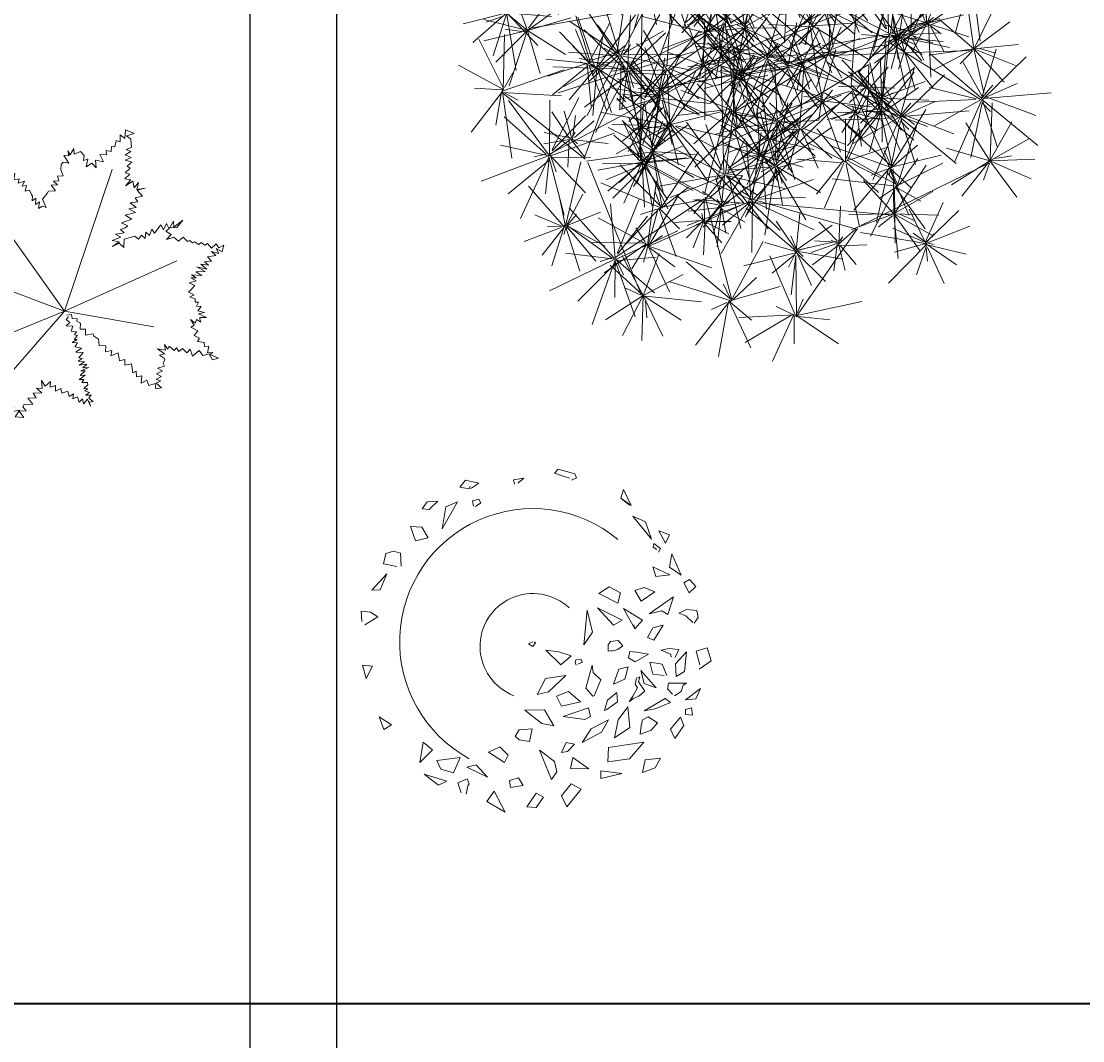
# Model space of a CAD drawing. Units: inches. Extents: x 8049 to 8459, y 820 to 1350.
# Tile 9 of 25: x 8132 to 8157, y 853 to 877. Entities that reach past the tile are written whole.
import ezdxf

# ---------------------------------------------------------------- set-up
doc = ezdxf.new("R2010")
doc.units = ezdxf.units.IN
doc.header["$MEASUREMENT"] = 0
for name, color, linetype, lineweight in [('A-ANNO-DIMS', 2, 'Continuous', 18), ('C-SITE-WALL', 7, 'Continuous', 35), ('zelen', 69, 'Continuous', 13)]:
    doc.layers.add(name, color=color, linetype=linetype, lineweight=lineweight)
doc.styles.get("Standard").update_dxf_attribs({"font": 'arial.ttf'})
doc.dimstyles.get("Standard").update_dxf_attribs({"dimtxt": 0.18, "dimasz": 0.18, "dimexe": 0.18, "dimexo": 0.0625, "dimgap": 0.09, "dimtad": 0, "dimtih": 1, "dimtoh": 1, "dimdec": 4, "dimzin": 0, "dimdsep": 46, "dimtxsty": 'Standard', "dimcen": 0.09, "dimadec": 0, "dimazin": 0, "dimtfac": 1, "dimtdec": 4, "dimtofl": 0, "dimtmove": 0, "dimatfit": 3, "dimfxl": 1, "dimtolj": 1, "dimtzin": 0, "dimarcsym": 0})

# ---------------------------------------------------------------- blocks, each defined once
blk = doc.blocks.new('z_96')
for p, q in [((-279.8, 149.9), (-254.2, 304.5)), ((-277.5, 143.8), (-209, 319.2)), ((0.6, 181.7), (29.5, 299.6)), ((-279.3, 139.9), (-326.8, 270.9)), ((-2.3, 183.5), (-55.4, 292.1)), ((5.7, 184.9), (91.8, 284.8)), ((-282.5, 143.4), (-440.4, 263.7)), ((1.7, 182.4), (-92.5, 262.1)), ((3.6, 188.7), (58.7, 265.3)), ((395.6, 94.6), (438.6, 246.5)), ((-276.5, 141.1), (-146.8, 221.3)), ((-9.6, 182.8), (-129.6, 222.9)), ((393.4, 89.6), (354, 209.2)), ((-292.1, 134.2), (-430.8, 180.4)), ((-5.7, 186.4), (-99.8, 114.3)), ((-4.6, 181.6), (-86.6, 72.3)), ((-0.6, 184.6), (125.7, 194.4)), ((1.5, 182.8), (69.9, 77.5)), ((9.8, 182.3), (88, 114.6)), ((393.4, 89.6), (479.1, 181.8)), ((-280.1, 150.3), (-304, 174)), ((-260.4, 142.3), (-97.9, 156.1)), ((-4.6, -3.2), (0.8, 176.4)), ((393.4, 89.6), (284.7, 153.1)), ((-283.2, 138.5), (-471.2, 114.9)), ((-279.1, 142.3), (-397.9, 16.9)), ((-285.6, 136.6), (-375, 92.2)), ((-277.6, 139.7), (-313.4, -1.1)), ((-279.1, 135.4), (-307.4, 99.5)), ((-278.4, 130.6), (-221.9, 40)), ((-277.5, 137.2), (-129.1, 19.3)), ((-17.8, -5.6), (-274.7, 141.8)), ((-263.2, 140.3), (-131, 113.5)), ((393.4, 89.6), (514.5, 123.6)), ((393.4, 89.6), (273.9, 50.1)), ((393.4, 89.6), (293.9, 12.5)), ((393.4, 89.6), (493.5, 13.4)), ((393.4, 89.6), (516.7, 64.5)), ((393.4, 89.6), (442.6, -26.2)), ((409.2, 93.4), (456.4, 89)), ((-71.7, -35.5), (-42.1, 65.4)), ((0, 0), (389.1, 84.4)), ((391.3, 83.5), (363.2, 41.9)), ((-74.7, -24.6), (-111.9, 37.5)), ((164.1, -89.9), (142.7, 11.7)), ((163.4, -89), (238.9, 7.6)), ((-237.5, -199.4), (-267, -22)), ((-10.4, -6), (-235.7, -205.3)), ((-65.2, -32.9), (-135.5, -11.4)), ((-80, -28.7), (-89.9, -20)), ((-16, -6.1), (-74.7, -37.4)), ((-68.1, -28.4), (-55.8, -19.3)), ((-5, -18.9), (163.8, -91.6)), ((159.3, -86.3), (85.5, -28.7)), ((167, -88.4), (276, -24.7)), ((-234, -202.3), (-196.3, -40.6)), ((-75, -39.2), (-157.1, -75.4)), ((-74, -33), (-152.4, -40.5)), ((-76.2, -35.8), (-103.5, -105.8)), ((-72.5, -35.1), (-71.9, -112)), ((-70.4, -41.1), (3.7, -57.1)), ((-69.9, -39.6), (-38.4, -102.6)), ((163.4, -86.5), (137.7, -55.7)), ((165.3, -92), (295.7, -74)), ((168.3, -88.4), (194, -71.5)), ((167.1, -94.6), (37.3, -175)), ((161.1, -92.4), (74, -95.2)), ((163.6, -101.8), (119, -170.9)), ((164.5, -93.4), (157.3, -141.4)), ((160.4, -93), (267.6, -148.2)), ((164.2, -92.2), (234.3, -170.2)), ((166.9, -90.5), (187.1, -100.1)), ((167, -104.1), (188, -212.9)), ((-237.4, -199.3), (-392.1, -169)), ((-246.4, -194), (-283.1, -163.8)), ((-231, -196), (-205.2, -161.9)), ((-242.3, -196.3), (-391.5, -241.3)), ((-242.2, -199.4), (-329.5, -310.3)), ((-241, -201.7), (-259.1, -277.3)), ((-242.2, -201.7), (-47.9, -207.3)), ((-236.2, -200.9), (-139.2, -306.8)), ((-230.8, -205.8), (-146.5, -236))]:
    blk.add_line(p, q)
blk = doc.blocks.new('сосна 1')
for p, rotation in [((317.7, 388.3), 121.1570021628385), ((-412.6, 386.5), 205.4822314301707), ((-117.1, 122.3), 55.05972244949475), ((-136.5, 361.1), 177.7388340989747), ((-351.5, 121.7), 257.3134436407499), ((-143.1, -5.5), 121.1570021628385), ((285.8, 9.1), 60.73020616460848), ((-343.1, -101.5), 57.88453704712605), ((234.4, -65.1), 73.8676290404427), ((-274, 161.3), 177.7388340989747), ((173.8, 17), 349.7944254651076), ((326.9, 45.9), 177.7388340989747), ((98.1, -4.6), 177.7388340989747), ((-175.3, -367), 63.19571700542104), ((-502.4, -282.3), 279.7984529833926), ((-48.9, -393.6), 342.5348703671633), ((260.9, -458.6), 13.72293452966709)]:
    blk.add_blockref('z_96', p, dxfattribs=dict(rotation=rotation))
blk = doc.blocks.new('z_85')
for p, q in [((168.5, 483.9), (169.7, 507.5)), ((169.7, 507.5), (194.7, 497.5)), ((140.4, 459.9), (144.1, 478.3)), ((144.1, 478.3), (154.8, 474.2)), ((154.8, 474.2), (155.6, 493.8)), ((155.6, 493.8), (168.5, 483.9)), ((194.7, 497.5), (173, 491.4)), ((173, 491.4), (185.2, 481.2)), ((185.2, 481.2), (186.9, 458.5)), ((8.4, 449), (15.4, 438)), ((11.7, 434.9), (8.4, 449)), ((15.4, 438), (25.6, 455.6)), ((25.6, 455.6), (26.4, 439.7)), ((26.4, 439.7), (44.1, 447.4)), ((44.1, 447.4), (54.4, 436.3)), ((116.1, 450.2), (130, 447.6)), ((116.6, 438), (116.1, 450.2)), ((130, 447.6), (130.9, 460.7)), ((130.9, 460.7), (140.4, 459.9)), ((185.1, 447.3), (169, 438)), ((186.9, 458.5), (172.1, 453.2)), ((172.1, 453.2), (185.1, 447.3)), ((-334.5, 433), (-320.5, 441.8)), ((-320.3, 426.3), (-334.5, 433)), ((-331, 417), (-320.3, 426.3)), ((-316.9, 407.2), (-331, 417)), ((-320.5, 441.8), (-312.2, 426.3)), ((-312.2, 426.3), (-302, 436.4)), ((-302, 436.4), (-292.5, 418.9)), ((-292.5, 418.9), (-282.7, 426.1)), ((-282.7, 426.1), (-277, 408.1)), ((-277, 408.1), (-266.3, 423.5)), ((-266.3, 423.5), (-258.7, 400.7)), ((-214.2, 421.3), (-198.5, 423)), ((-207.8, 406.4), (-214.2, 421.3)), ((-198.5, 423), (-198.2, 434.1)), ((-198.2, 434.1), (-192.6, 433.8)), ((-192.6, 433.8), (-192.5, 442.2)), ((-192.5, 442.2), (-183.3, 424.5)), ((-183.3, 424.5), (-173.3, 433.2)), ((-173.3, 433.2), (-176.4, 415.5)), ((-176.4, 415.5), (-165.1, 418.9)), ((-165.1, 418.9), (-166.4, 400.3)), ((-9.6, 410.9), (-3.8, 416.9)), ((-3.8, 416.9), (11.4, 414.5)), ((-2.1, 435.8), (11.7, 434.9)), ((11.4, 414.5), (-2.1, 435.8)), ((54.4, 436.3), (52.3, 421.7)), ((52.3, 421.7), (64.6, 426)), ((64.6, 426), (59.8, 403.9)), ((86.4, 422.5), (108.9, 418.4)), ((88.3, 401.4), (86.4, 422.5)), ((98.5, 438.8), (116.6, 438)), ((108.9, 418.4), (98.5, 438.8)), ((169, 438), (186.4, 430.3)), ((186.4, 430.3), (169.1, 422.7)), ((169.1, 422.7), (188.1, 417.5)), ((188.1, 417.5), (174.5, 406.5)), ((-325.3, 394.5), (-316.9, 407.2)), ((-309.5, 388.7), (-325.3, 394.5)), ((-317.2, 380.4), (-309.5, 388.7)), ((-258.7, 400.7), (-250.8, 414.2)), ((-250.8, 414.2), (-244.9, 399.8)), ((-244.9, 399.8), (-237.2, 410.8)), ((-237.2, 410.8), (-228.5, 393.9)), ((-228.5, 393.9), (-223.5, 408.6)), ((-223.5, 408.6), (-207.8, 406.4)), ((-166.4, 400.3), (-152.4, 402.8)), ((-152.4, 402.8), (-154.8, 385.2)), ((-10.8, 396), (-9.6, 410.9)), ((-4.1, 379.1), (-10.8, 396)), ((0, 0), (132.7, 397)), ((59.8, 403.9), (75.6, 414.2)), ((75.6, 414.2), (88.3, 401.4)), ((183.6, 400.7), (169.1, 387.1)), ((169.1, 387.1), (182.7, 383.5)), ((174.5, 406.5), (183.6, 400.7)), ((-305.1, 378.2), (-317.2, 380.4)), ((-309.5, 366.8), (-305.1, 378.2)), ((-299.2, 360.3), (-309.5, 366.8)), ((-305.9, 349.8), (-299.2, 360.3)), ((-154.8, 385.2), (-139.8, 385.6)), ((-139.8, 385.6), (-142, 367.5)), ((-142, 367.5), (-126.8, 370.7)), ((-126.8, 370.7), (-129.7, 358.9)), ((-129.7, 358.9), (-112.6, 364.1)), ((-112.6, 364.1), (-118.7, 349.7)), ((-31.2, 364.3), (-16.4, 364.7)), ((-19.6, 354.2), (-31.2, 364.3)), ((-19.9, 378.2), (-4.1, 379.1)), ((-16.4, 364.7), (-19.9, 378.2)), ((182.7, 383.5), (168.5, 371)), ((168.5, 371), (185.5, 367.5)), ((185.5, 367.5), (169.7, 351.3)), ((169.7, 351.3), (191.1, 364.1)), ((191.1, 364.1), (194, 345.3)), ((194, 345.3), (206.3, 360.8)), ((206.3, 360.8), (201.7, 341.2)), ((-292.6, 345.9), (-305.9, 349.8)), ((-305.3, 333.9), (-292.6, 345.9)), ((-288.9, 332.3), (-305.3, 333.9)), ((-296.8, 323.1), (-288.9, 332.3)), ((0, 0), (-245.8, 345.3)), ((-118.7, 349.7), (-106.5, 351.7)), ((-106.5, 351.7), (-110.4, 335.8)), ((-110.4, 335.8), (-98.6, 339.2)), ((-98.6, 339.2), (-92.9, 326.8)), ((-92.9, 326.8), (-89.6, 322.3)), ((-61.6, 314), (-48.8, 329.6)), ((-48.8, 329.6), (-45, 336.2)), ((-45, 336.2), (-26.1, 337)), ((-37.5, 352.7), (-19.6, 354.2)), ((-26.1, 337), (-37.5, 352.7)), ((201.7, 341.2), (224.8, 344.2)), ((224.8, 344.2), (203.2, 339.2)), ((203.2, 339.2), (217.5, 321.8)), ((-348.8, 287.5), (-334.3, 298.5)), ((-334.3, 298.5), (-333.4, 308.7)), ((-333.4, 308.7), (-315.2, 298.3)), ((-315.2, 298.3), (-314.9, 314.1)), ((-314.9, 314.1), (-305, 309.4)), ((-305, 309.4), (-300.9, 321)), ((-300.9, 321), (-284.3, 312.7)), ((-283.1, 324), (-296.8, 323.1)), ((-284.3, 312.7), (-283.1, 324)), ((-89.6, 322.3), (-91.1, 309)), ((-91.1, 309), (-80.4, 316.3)), ((-80.4, 316.3), (-81.2, 298.5)), ((-81.2, 298.5), (-70.2, 306.6)), ((-70.2, 306.6), (-73.6, 287.8)), ((-51.7, 290.2), (-61.6, 314)), ((204.7, 306.3), (183.1, 303.2)), ((183.1, 303.2), (199.8, 290.5)), ((217.5, 321.8), (196.8, 317.3)), ((196.8, 317.3), (204.7, 306.3)), ((-329.7, 291.9), (-348.8, 287.5)), ((-335.7, 285.2), (-329.7, 291.9)), ((-323.9, 282.5), (-335.7, 285.2)), ((-327.7, 273.4), (-323.9, 282.5)), ((-312.5, 269.8), (-327.7, 273.4)), ((-318.1, 260.9), (-312.5, 269.8)), ((-73.6, 287.8), (-62, 294.6)), ((-62, 294.6), (-51.7, 290.2)), ((198, 276.2), (169.3, 269.4)), ((169.3, 269.4), (187.9, 258.2)), ((199.8, 290.5), (179.5, 286.4)), ((179.5, 286.4), (198, 276.2)), ((-386.6, 246.8), (-370.9, 243.8)), ((-380.3, 234.1), (-386.6, 246.8)), ((-370.9, 243.8), (-362.5, 240.1)), ((-362.5, 240.1), (-355.4, 227.7)), ((-303.5, 257.1), (-318.1, 260.9)), ((-306.9, 250.2), (-303.5, 257.1)), ((-296.5, 245.4), (-306.9, 250.2)), ((-304.8, 236.9), (-296.5, 245.4)), ((187.9, 258.2), (158.6, 247.3)), ((158.6, 247.3), (176.5, 239.3)), ((176.5, 239.3), (169.1, 234)), ((251.2, 218.3), (269.1, 241.8)), ((269.1, 241.8), (276.1, 228.2)), ((276.1, 228.2), (284.6, 245.4)), ((284.6, 245.4), (292.5, 230.8)), ((292.5, 230.8), (304.2, 252.6)), ((304.2, 252.6), (305.4, 235.8)), ((305.4, 235.8), (330.6, 255.3)), ((330.6, 255.3), (314, 234.4)), ((-392, 203.9), (-391, 210.5)), ((-391, 210.5), (-375.1, 210.9)), ((-387.5, 216.4), (-377.3, 224.9)), ((-375.1, 210.9), (-387.5, 216.4)), ((-387.2, 228.2), (-380.3, 234.1)), ((-377.3, 224.9), (-387.2, 228.2)), ((-355.4, 227.7), (-347.7, 237.1)), ((-347.7, 237.1), (-340.1, 223.9)), ((-340.1, 223.9), (-331.2, 232.1)), ((-331.2, 232.1), (-323, 219.9)), ((-323, 219.9), (-314.9, 229.4)), ((-314.9, 229.4), (-308.7, 210.5)), ((-308.7, 210.5), (-301.4, 220.5)), ((-284, 230.8), (-304.8, 236.9)), ((-301.4, 220.5), (-296.2, 209.5)), ((-296.2, 209.5), (-288.7, 218.5)), ((-288.7, 218.5), (-282.8, 208)), ((-287.5, 222.7), (-284, 230.8)), ((-267.9, 221.3), (-287.5, 222.7)), ((-282.8, 208), (-278.3, 215.3)), ((-278.3, 215.3), (-269.6, 197)), ((-272.7, 208.1), (-267.9, 221.3)), ((-249.1, 208.6), (-272.7, 208.1)), ((-252.6, 191.1), (-249.1, 208.6)), ((166.6, 220), (142.5, 215.8)), ((142.5, 215.8), (157.5, 207.7)), ((169.1, 234), (156.5, 228.6)), ((156.5, 228.6), (166.6, 220)), ((166.1, 202.2), (195.8, 210)), ((195.8, 210), (206.3, 202.3)), ((206.3, 202.3), (214.9, 212.7)), ((214.9, 212.7), (225, 203.7)), ((225, 203.7), (227.4, 221.4)), ((227.4, 221.4), (237.6, 211.9)), ((237.6, 211.9), (244, 229.6)), ((244, 229.6), (251.2, 218.3)), ((291.9, 231.3), (282.8, 224.3)), ((282.8, 224.3), (297.7, 215.3)), ((297.7, 215.3), (285.2, 201.4)), ((294, 233.8), (291.9, 231.3)), ((314, 234.4), (294, 233.8)), ((-547.4, 195.4), (-527.9, 192.6)), ((-544.7, 179.5), (-547.4, 195.4)), ((-524.7, 189.5), (-544.7, 179.5)), ((-528.5, 176.6), (-524.7, 189.5)), ((-527.9, 192.6), (-523, 206.4)), ((-523, 206.4), (-504.7, 194.2)), ((-504.7, 194.2), (-496.5, 204.8)), ((-496.5, 204.8), (-486, 196.2)), ((-486, 196.2), (-473.8, 197.3)), ((-473.8, 197.3), (-470.6, 205)), ((-470.6, 205), (-459, 197.9)), ((-459, 197.9), (-453.2, 204.7)), ((-453.2, 204.7), (-441.7, 197.3)), ((-441.7, 197.3), (-436, 206.1)), ((-436, 206.1), (-423, 196.7)), ((-423, 196.7), (-417.9, 205.5)), ((-417.9, 205.5), (-411.3, 200.8)), ((-411.3, 200.8), (-403.9, 207.3)), ((-403.9, 207.3), (-392, 203.9)), ((-269.6, 197), (-261.6, 206.7)), ((-261.6, 206.7), (-252.6, 191.1)), ((157.5, 207.7), (133, 198.3)), ((133, 198.3), (152.7, 194.8)), ((152.7, 194.8), (134.2, 181.8)), ((134.2, 181.8), (152.3, 190.3)), ((152.3, 190.3), (165.5, 178.4)), ((165.5, 178.4), (166.1, 202.2)), ((285.2, 201.4), (305.7, 207.8)), ((305.7, 207.8), (318.4, 196.7)), ((318.4, 196.7), (331.5, 207.2)), ((331.5, 207.2), (343.4, 195.3)), ((343.4, 195.3), (349.2, 197.8)), ((349.2, 197.8), (357.1, 191.7)), ((357.1, 191.7), (363.4, 194)), ((363.4, 194), (375.4, 187.3)), ((375.4, 187.3), (381.6, 192.9)), ((381.6, 192.9), (391.6, 185.1)), ((391.6, 185.1), (399.5, 189.8)), ((399.5, 189.8), (410.7, 177.1)), ((410.7, 177.1), (423.8, 189)), ((423.8, 189), (430.9, 177.3)), ((430.9, 177.3), (445.2, 185.4)), ((445.2, 185.4), (440.2, 166.6)), ((-515.5, 177.6), (-528.5, 176.6)), ((-516.7, 167.9), (-515.5, 177.6)), ((-506.3, 173.2), (-516.7, 167.9)), ((-504.7, 162.4), (-506.3, 173.2)), ((-491.4, 165.7), (-504.7, 162.4)), ((-484.9, 140.6), (-491.4, 165.7)), ((0, 0), (-394.4, 149.4)), ((422.9, 156), (399.8, 152.7)), ((399.8, 152.7), (410.7, 140.5)), ((410.7, 167.7), (422.9, 156)), ((431.6, 161.5), (410.7, 167.7)), ((423.8, 175.6), (431.6, 161.5)), ((440.2, 166.6), (423.8, 175.6)), ((-472, 147), (-484.9, 140.6)), ((-466.4, 131.1), (-472, 147)), ((-447.4, 143.9), (-466.4, 131.1)), ((-446.4, 127.5), (-447.4, 143.9)), ((-431.2, 136.1), (-446.4, 127.5)), ((-433.6, 116.8), (-432.5, 124.7)), ((-432.5, 124.7), (-431.2, 136.1)), ((0, 0), (313.9, 140.8)), ((370, 124.5), (392.9, 111.3)), ((397.4, 117.9), (370, 124.5)), ((380.7, 131.9), (397.4, 117.9)), ((402.3, 129), (380.7, 131.9)), ((410.7, 140.5), (391.1, 138)), ((391.1, 138), (402.3, 129)), ((-456.8, 97.3), (-437.9, 103.7)), ((-452.6, 88.2), (-456.8, 97.3)), ((-447.3, 109), (-420.9, 115.7)), ((-437.9, 103.7), (-447.3, 109)), ((-420.9, 115.7), (-433.6, 116.8)), ((367.3, 93.6), (352.7, 93.5)), ((352.7, 93.5), (367.5, 85.5)), ((354.4, 102.3), (367.3, 93.6)), ((384, 100.5), (354.4, 102.3)), ((392.9, 111.3), (367, 110.4)), ((367, 110.4), (384, 100.5)), ((-490.1, 61.5), (-485.7, 76.6)), ((-472.7, 67.7), (-490.1, 61.5)), ((-485.7, 76.6), (-461.1, 77.2)), ((-477.3, 56.2), (-472.7, 67.7)), ((-464.1, 63.3), (-477.3, 56.2)), ((-468.4, 52.6), (-464.1, 63.3)), ((-452, 61.1), (-468.4, 52.6)), ((-466.3, 86.6), (-452.6, 88.2)), ((-461.1, 77.2), (-466.3, 86.6)), ((-455.1, 51.2), (-452, 61.1)), ((-439, 59.8), (-455.1, 51.2)), ((-439.5, 47.5), (-439, 59.8)), ((355.3, 62.8), (346.4, 53.6)), ((367.5, 85.5), (348.2, 79.7)), ((348.2, 79.7), (364, 72.5)), ((364, 72.5), (355.3, 62.8)), ((-428.5, 56.1), (-439.5, 47.5)), ((-421.5, 42.4), (-428.5, 56.1)), ((-408.4, 49.5), (-421.5, 42.4)), ((-406.6, 37.3), (-408.4, 49.5)), ((-393.5, 46.8), (-406.6, 37.3)), ((-392.2, 37), (-393.5, 46.8)), ((-375.3, 43.4), (-392.2, 37)), ((-368.7, 27.4), (-375.3, 43.4)), ((-356.3, 36.3), (-368.7, 27.4)), ((-348.5, 20.8), (-356.3, 36.3)), ((-333.9, 32.3), (-348.5, 20.8)), ((-335.5, 21.5), (-333.9, 32.3)), ((346.4, 53.6), (362.3, 46.4)), ((362.3, 46.4), (350.4, 40.1)), ((350.4, 40.1), (365.4, 35.2)), ((365.4, 35.2), (364.6, 26)), ((-322.4, 29.1), (-335.5, 21.5)), ((-319.9, 12.2), (-322.4, 29.1)), ((-303.8, 20), (-319.9, 12.2)), ((0, 0), (-312.2, -125)), ((-297.7, 5.3), (-303.8, 20)), ((-284.2, 12.8), (-297.7, 5.3)), ((-282.8, 2.5), (-284.2, 12.8)), ((-266.1, 11.6), (-282.8, 2.5)), ((-268.5, 0.9), (-266.1, 11.6)), ((-245.2, 1.9), (-268.5, 0.9)), ((-258.6, 1.3), (-245.2, 1.9)), ((-256.6, -5.5), (-258.6, 1.3)), ((0, 0), (-163.1, -186)), ((0, 0), (249.7, -43.2)), ((364.6, 26), (373.9, 25.2)), ((373.9, 25.2), (368.8, 14.6)), ((368.8, 14.6), (381.5, 13.5)), ((381.5, 13.5), (372.3, 1.1)), ((372.3, 1.1), (390.8, -3.1)), ((-337, -39.8), (-335.4, -26.5)), ((-335.4, -26.5), (-320, -32.7)), ((-320, -32.7), (-316.6, -19.6)), ((-316.6, -19.6), (-303.5, -24.4)), ((-303.5, -24.4), (-299.1, -12.1)), ((-299.1, -12.1), (-288.4, -18.9)), ((-288.4, -18.9), (-284.9, -7.8)), ((-284.9, -7.8), (-270.6, -10.5)), ((-272, -3.8), (-256.6, -5.5)), ((-270.6, -10.5), (-272, -3.8)), ((11, -15.5), (4.4, -23.3)), ((4.4, -23.3), (14.2, -31.5)), ((19.4, -9.1), (6, -11.1)), ((20.6, -19.7), (19.4, -9.1)), ((34.5, -21), (20.6, -19.7)), ((33.9, -27.7), (34.5, -21)), ((44.7, -33.5), (33.9, -27.7)), ((352.1, -22.6), (362.5, -39.2)), ((365.2, -32.7), (352.1, -22.6)), ((368.7, -23.2), (365.2, -32.7)), ((380.7, -30.1), (368.7, -23.2)), ((390.8, -3.1), (374.2, -7.2)), ((374.2, -7.2), (396.2, -16.9)), ((378.3, -17.7), (377.9, -21.9)), ((377.9, -21.9), (380.7, -30.1)), ((396.2, -16.9), (378.3, -17.7)), ((-423.6, -64.7), (-418.1, -55.3)), ((-418.1, -55.3), (-406.6, -63.9)), ((-406.6, -63.9), (-402.1, -52.8)), ((-402.1, -52.8), (-387.5, -58.3)), ((-387.5, -58.3), (-386, -47.3)), ((-386, -47.3), (-378.3, -50.6)), ((-378.3, -50.6), (-371.8, -40.4)), ((-371.8, -40.4), (-358.3, -47.6)), ((-358.6, -35.2), (-337, -39.8)), ((-358.3, -47.6), (-358.6, -35.2)), ((14.2, -31.5), (3.8, -40.4)), ((3.8, -40.4), (23.3, -42)), ((23.3, -42), (17.8, -55.3)), ((17.8, -55.3), (33.3, -57.2)), ((33.3, -57.2), (27.6, -66.1)), ((43.2, -50.4), (44.7, -33.5)), ((57.8, -49.8), (43.2, -50.4)), ((57.8, -66.7), (57.8, -49.8)), ((362.5, -39.2), (352.9, -44.5)), ((352.9, -44.5), (372.4, -54.8)), ((372.4, -54.8), (362.2, -67.3)), ((-445.6, -85.2), (-442.8, -66.9)), ((-431.8, -81.7), (-445.6, -85.2)), ((-442.8, -66.9), (-423.6, -64.7)), ((-433, -93.3), (-431.8, -81.7)), ((-421.5, -86.1), (-433, -93.3)), ((-420.3, -102.3), (-421.5, -86.1)), ((35.4, -79.2), (20.9, -86.9)), ((20.9, -86.9), (36.1, -88.5)), ((35.8, -67.3), (26.2, -78.5)), ((26.2, -78.5), (35.4, -79.2)), ((27.6, -66.1), (35.8, -67.3)), ((36.1, -88.5), (28.2, -99.3)), ((79.4, -63.3), (57.8, -66.7)), ((80.6, -68.6), (79.4, -63.3)), ((95, -77.7), (80.6, -68.6)), ((96.5, -95.7), (95, -77.7)), ((362.2, -67.3), (377.4, -74.9)), ((377.4, -74.9), (371.4, -84.3)), ((371.4, -84.3), (390.2, -87.1)), ((390.2, -87.1), (391, -98.7)), ((-408.9, -93.6), (-420.3, -102.3)), ((-406.5, -108.7), (-408.9, -93.6)), ((-396.2, -96.8), (-406.5, -108.7)), ((-391.4, -111), (-396.2, -96.8)), ((-377.3, -108.5), (-391.4, -111)), ((-387.6, -122.5), (-377.3, -108.5)), ((28.2, -99.3), (46.8, -102.9)), ((31.9, -112.9), (31.3, -114)), ((31.3, -114), (51.4, -114.8)), ((46.8, -102.9), (31.9, -112.9)), ((51.4, -114.8), (39.8, -130.3)), ((114.9, -96.9), (96.5, -95.7)), ((113.9, -113.2), (114.9, -96.9)), ((131.6, -109.3), (113.9, -113.2)), ((129.5, -124.2), (131.6, -109.3)), ((150, -116), (129.5, -124.2)), ((153.5, -138.6), (150, -116)), ((259.9, -104.5), (278.9, -118.5)), ((281.6, -108.4), (259.9, -104.5)), ((278.9, -118.5), (264.8, -122.8)), ((279.1, -92.7), (281.6, -108.4)), ((288.4, -105.6), (279.1, -92.7)), ((292.3, -97.7), (288.4, -105.6)), ((306.3, -109.8), (292.3, -97.7)), ((312.3, -101.9), (306.3, -109.8)), ((319.1, -112.6), (312.3, -101.9)), ((329.4, -104.1), (319.1, -112.6)), ((341.7, -115.9), (329.4, -104.1)), ((350.6, -106.3), (341.7, -115.9)), ((357.5, -125.6), (350.6, -106.3)), ((375.9, -109.5), (357.5, -125.6)), ((386.6, -123.9), (375.9, -109.5)), ((403.8, -118.5), (386.6, -123.9)), ((391, -98.7), (403.6, -97.7)), ((403.6, -97.7), (399.4, -115.7)), ((399.4, -115.7), (414.2, -115.6)), ((413.1, -135.8), (403.8, -118.5)), ((414.2, -115.6), (406.2, -120.7)), ((-399.4, -144.9), (-386, -138.6)), ((-391.7, -153.5), (-399.4, -144.9)), ((-396.7, -133.3), (-378.8, -121.8)), ((-386, -138.6), (-396.7, -133.3)), ((-378.8, -121.8), (-387.6, -122.5)), ((49.4, -132), (38, -139.7)), ((38, -139.7), (55.7, -140.9)), ((39.8, -130.3), (49.4, -132)), ((55.7, -140.9), (40.8, -150.5)), ((40.8, -150.5), (61.7, -147.7)), ((61.7, -147.7), (51.2, -158.2)), ((168.2, -134.7), (153.5, -138.6)), ((168.7, -151.1), (168.2, -134.7)), ((187.2, -147), (168.7, -151.1)), ((190.4, -171.9), (187.2, -147)), ((264.8, -122.8), (279.4, -131.9)), ((280.4, -134.4), (275.3, -145.6)), ((275.3, -145.6), (279.5, -153.9)), ((279.4, -131.9), (280.4, -134.4)), ((406.2, -120.7), (430, -130.9)), ((430, -130.9), (413.1, -135.8)), ((-407.1, -178.7), (-394, -170.7)), ((-405.7, -161.9), (-391.7, -153.5)), ((-394, -170.7), (-405.7, -161.9)), ((57.7, -166.9), (43.5, -179.6)), ((67.9, -157.4), (45.5, -166.6)), ((45.5, -166.6), (57.7, -166.9)), ((51.2, -158.2), (67.9, -157.4)), ((199.5, -167.6), (190.4, -171.9)), ((201.2, -183.5), (199.5, -167.6)), ((273.9, -166.2), (257.2, -175.1)), ((257.2, -175.1), (270.6, -182.1)), ((279.5, -153.9), (259.5, -159.1)), ((259.5, -159.1), (273.9, -166.2)), ((-408.7, -191.2), (-407.1, -178.7)), ((-386.3, -183.7), (-408.7, -191.2)), ((-386.9, -194.2), (-386.3, -183.7)), ((-375, -185.4), (-386.9, -194.2)), ((-374.4, -200.4), (-375, -185.4)), ((-361, -190), (-374.4, -200.4)), ((-355.6, -205.5), (-361, -190)), ((-340.1, -188.9), (-355.6, -205.5)), ((-331, -204.2), (-340.1, -188.9)), ((-320.5, -190.1), (-331, -204.2)), ((-315.8, -206.4), (-320.5, -190.1)), ((-300.9, -199.4), (-315.8, -206.4)), ((-311, -217.5), (-300.9, -199.4)), ((-64.5, -193.4), (-63.1, -216.4)), ((-54.1, -209.7), (-64.5, -193.4)), ((-39.9, -196.5), (-54.1, -209.7)), ((-40.4, -212.5), (-39.9, -196.5)), ((-25.3, -207.7), (-40.4, -212.5)), ((-25.3, -223.8), (-25.3, -207.7)), ((57.1, -178.7), (40.5, -191.1)), ((40.5, -191.1), (53.9, -190.4)), ((43.5, -179.6), (57.1, -178.7)), ((53.9, -190.4), (47.9, -199)), ((47.9, -199), (63.4, -198.7)), ((65.1, -205.6), (53.6, -216.1)), ((63.4, -198.7), (65.1, -205.6)), ((215.4, -180.2), (201.2, -183.5)), ((214.3, -200.6), (215.4, -180.2)), ((229.7, -192.5), (214.3, -200.6)), ((235.5, -207.5), (229.7, -192.5)), ((253.5, -202), (235.5, -207.5)), ((255.4, -217.1), (253.5, -202)), ((270.6, -182.1), (255.6, -190.7)), ((255.6, -190.7), (268.7, -194.5)), ((268.7, -194.5), (256, -201.4)), ((256, -201.4), (270.6, -214.1)), ((-316.4, -230.7), (-301.2, -212.5)), ((-303, -227.7), (-316.4, -230.7)), ((-301.2, -212.5), (-311, -217.5)), ((-309.9, -238.3), (-303, -227.7)), ((-63.4, -228.2), (-87.9, -229.1)), ((-87.9, -229.1), (-79.8, -242)), ((-78.5, -215.2), (-63.4, -228.2)), ((-63.1, -216.4), (-78.5, -215.2)), ((-10.7, -215.8), (-25.3, -223.8)), ((-8.3, -228.6), (-10.7, -215.8)), ((8.9, -223.5), (-8.3, -228.6)), ((12.7, -238.7), (8.9, -223.5)), ((24.7, -230.5), (12.7, -238.7)), ((23, -244.8), (24.7, -230.5)), ((53.6, -216.1), (64.9, -216.9)), ((64.9, -216.9), (56, -222.4)), ((56, -222.4), (69.4, -226.9)), ((69.4, -226.9), (58.1, -234.3)), ((58.1, -234.3), (70.9, -234.4)), ((73.9, -233.5), (67.9, -243.4)), ((70.9, -234.4), (73.9, -233.5)), ((270.6, -214.1), (255.4, -217.1)), ((-298.3, -242.6), (-309.9, -238.3)), ((-305.3, -270.9), (-295, -254.3)), ((-304.7, -251.3), (-298.3, -242.6)), ((-295, -254.3), (-304.7, -251.3)), ((-166.3, -266.5), (-182.4, -271.4)), ((-151.2, -278.6), (-166.3, -266.5)), ((-113.1, -261.1), (-117.3, -267.5)), ((-88.9, -260), (-113.1, -261.1)), ((-79.8, -242), (-103.3, -242.6)), ((-103.3, -242.6), (-88.9, -260)), ((35.5, -238.8), (23, -244.8)), ((40.7, -254.5), (35.5, -238.8)), ((49.8, -244.9), (40.7, -254.5)), ((52.7, -259.2), (49.8, -244.9)), ((63.6, -245.9), (52.7, -259.2)), ((72.4, -265), (63.6, -245.9)), ((67.9, -243.4), (79.4, -252.4)), ((79.4, -252.4), (68.2, -253.9)), ((68.2, -253.9), (72.4, -265)), ((-290.1, -273.1), (-305.3, -270.9)), ((-294.6, -284.2), (-290.1, -273.1)), ((-277.1, -277.7), (-294.6, -284.2)), ((-264.9, -273), (-283.1, -288.1)), ((-283.1, -288.1), (-277.1, -277.7)), ((-264.3, -294.3), (-264.9, -273)), ((-256.6, -277.5), (-264.3, -294.3)), ((-254.5, -286.6), (-256.6, -277.5)), ((-239.6, -270.1), (-254.5, -286.6)), ((-228.6, -289.1), (-239.6, -270.1)), ((-220, -272), (-228.6, -289.1)), ((-197.9, -289.9), (-220, -272)), ((-199.2, -272), (-197.9, -289.9)), ((-184.2, -282), (-199.2, -272)), ((-182.4, -271.4), (-184.2, -282)), ((-142.3, -267.5), (-151.2, -278.6)), ((-144.6, -280.3), (-142.3, -267.5)), ((-126.2, -276.2), (-144.6, -280.3)), ((-138.9, -294.9), (-126.2, -276.2)), ((-114.3, -296.8), (-138.9, -294.9)), ((-107.8, -278), (-127.3, -279.2)), ((-127.3, -279.2), (-114.3, -296.8)), ((-117.3, -267.5), (-107.8, -278))]:
    blk.add_line(p, q)
blk = doc.blocks.new('z_66')
for p, q in [((83.2, 488.9), (72.7, 477.7)), ((72.7, 477.7), (96.4, 469.7)), ((129.8, 476.2), (83.2, 488.9)), ((134, 464.6), (129.8, 476.2)), ((-176.4, 458.5), (-191.7, 438.6)), ((-139.2, 449.4), (-176.4, 458.5)), ((-161.1, 434.6), (-139.2, 449.4)), ((-13.6, 463.6), (-42.5, 459.2)), ((-42.5, 459.2), (-39.3, 446.9)), ((-30.3, 449.4), (-13.6, 463.6)), ((96.4, 469.7), (114.5, 463.9)), ((114.5, 463.9), (114.5, 463.9)), ((120.4, 457.8), (134, 464.6)), ((-191.7, 438.6), (-165.6, 433.5)), ((-165.6, 433.5), (-163.6, 441.1)), ((-165.6, 433.5), (-165.6, 433.5)), ((265.2, 432.1), (258.2, 407.5)), ((287.4, 387.2), (265.2, 432.1)), ((-283.6, 397.7), (-297.2, 378.2)), ((-254, 399.9), (-283.6, 397.7)), ((-272.8, 380.7), (-254, 399.9)), ((-241.9, 321.7), (-199.1, 397.3)), ((-199.1, 397.3), (-231.4, 383.6)), ((-138.9, 404.9), (-156.9, 400.2)), ((-156.9, 400.2), (-153.8, 385.4)), ((-148.6, 384.7), (-133.3, 394.8)), ((-133.3, 394.8), (-138.9, 404.9)), ((258.2, 407.5), (287.4, 387.2)), ((258.2, 407.5), (281.9, 388.6)), ((281.9, 388.6), (281.9, 388.6)), ((-297.2, 378.2), (-277.7, 376)), ((-277.7, 376), (-272.8, 380.7)), ((-231.4, 383.6), (-241.9, 321.7)), ((344.2, 293.1), (292, 357.2)), ((292, 357.2), (326.8, 341.2)), ((-330.3, 328.9), (-298.6, 327.1)), ((-316, 288.8), (-330.3, 328.9)), ((-298.6, 327.1), (-280.8, 297.1)), ((326.8, 341.2), (344.2, 293.1)), ((-280.8, 297.1), (-316, 288.8)), ((383.1, 281.9), (364.4, 316.3)), ((364.4, 316.3), (394.6, 305.1)), ((394.6, 305.1), (383.1, 281.9)), ((350.8, 280.8), (348.7, 270.3)), ((348.7, 270.3), (358.8, 264.5)), ((369.2, 266.7), (350.8, 280.8)), ((-399.2, 252.6), (-405.8, 224)), ((-377.9, 259.1), (-399.2, 252.6)), ((-358.4, 254), (-377.9, 259.1)), ((-356, 217.5), (-358.4, 254)), ((358.8, 264.5), (358.8, 264.5)), ((363.3, 256.6), (369.2, 266.7)), ((400.9, 251.9), (393.9, 214.6)), ((426.6, 192.2), (400.9, 251.9)), ((-405.8, 224), (-368.2, 216.4)), ((-368.2, 216.4), (-368.2, 216.4)), ((348, 215.7), (356, 188.9)), ((395.3, 193.2), (348, 215.7)), ((393.9, 214.6), (426.6, 192.2)), ((-396.4, 196.1), (-438.1, 150.2)), ((-414.8, 150.9), (-396.4, 196.1)), ((356, 188.9), (395.3, 193.2)), ((450, 180.6), (434.3, 171.2)), ((467.7, 160.3), (450, 180.6)), ((-438.1, 150.2), (-414.8, 150.9)), ((225.2, 159.9), (197, 140.8)), ((256.8, 142.6), (225.2, 159.9)), ((323.6, 157.8), (297.5, 149.8)), ((297.5, 149.8), (314.6, 119.4)), ((352.9, 145.5), (323.6, 157.8)), ((434.3, 171.2), (449.6, 142.6)), ((449.6, 142.6), (467.7, 160.3)), ((197, 140.8), (249.5, 113.6)), ((249.5, 113.6), (256.8, 142.6)), ((314.6, 119.4), (352.9, 145.5)), ((336.9, 84.3), (405.8, 131.7)), ((405.8, 131.7), (389.8, 82.1)), ((-468.4, 91.6), (-466.3, 62.6)), ((-441.6, 89), (-468.4, 91.6)), ((164.3, 94.8), (154.2, -2.2)), ((178.9, 33.3), (164.3, 94.8)), ((193.1, 101.3), (238, 52.1)), ((261.7, 66.6), (193.1, 101.3)), ((265.2, 98.8), (297.2, 42.7)), ((318.8, 66.2), (265.2, 98.8)), ((372.7, 93), (336.9, 84.3)), ((389.8, 82.1), (372.7, 93)), ((441.6, 95.9), (420.7, 86.5)), ((470.5, 93.7), (441.6, 95.9)), ((474, 73.5), (470.5, 93.7)), ((-466.3, 62.6), (-466.3, 62.6)), ((-458.3, 53.9), (-421.1, 76)), ((-421.1, 76), (-441.6, 89)), ((238, 52.1), (261.7, 66.6)), ((297.2, 42.7), (318.8, 66.2)), ((420.7, 86.5), (440.2, 78.5)), ((440.2, 78.5), (459.7, 59.7)), ((459.7, 59.7), (459.7, 59.7)), ((463.2, 57.9), (474, 73.5)), ((154.2, -2.2), (178.9, 33.3)), ((297.2, 42.7), (294.1, 53.6)), ((347.3, 45.2), (332.7, 18.1)), ((376.9, 52.5), (347.3, 45.2)), ((350.8, 10.9), (376.9, 52.5)), ((11.8, 6.2), (0, 0)), ((0, 0), (12.2, -6.9)), ((12.2, -6.9), (19.1, 2.9)), ((19.1, 2.9), (15.7, 5.8)), ((229, 7.2), (223.1, -2.5)), ((250.6, 9.8), (229, 7.2)), ((263.4, -5.4), (250.6, 9.8)), ((332.7, 18.1), (350.8, 10.9)), ((84.6, -21.7), (48, -17)), ((48, -17), (90.1, -58.3)), ((119.4, -32.9), (84.6, -21.7)), ((223.1, -2.5), (222.7, -20.6)), ((222.7, -20.6), (234.2, -18.1)), ((233.2, -19.9), (249.9, -15.9)), ((234.2, -18.1), (234.2, -18.1)), ((249.9, -15.9), (263.4, -5.4)), ((282.9, -21.3), (279.1, -39.1)), ((302.1, -22.8), (282.9, -21.3)), ((298.6, -50.3), (335.8, -28.6)), ((335.8, -28.6), (302.1, -22.8)), ((393.6, -13), (371, -17)), ((371, -17), (383.5, -23.5)), ((383.5, -23.5), (396.7, -28.9)), ((420, -15.9), (393.6, -13)), ((396.7, -28.9), (398.5, -35.5)), ((410.3, -38), (420, -15.9)), ((442, -22.4), (411.3, -55.4)), ((436, -77.1), (442, -22.4)), ((499.7, -10.9), (468.8, -19.9)), ((468.8, -19.9), (478.8, -58.6)), ((510.9, -47), (499.7, -10.9)), ((-464.2, -59.3), (-436.4, -62.6)), ((-454.5, -96.3), (-464.2, -59.3)), ((90.1, -58.3), (119.4, -32.9)), ((131.9, -44.9), (130.2, -52.5)), ((130.2, -52.5), (132.9, -59.3)), ((146.5, -42.3), (131.9, -44.9)), ((138.2, -56.8), (151, -51)), ((151, -51), (146.5, -42.3)), ((177.8, -59), (160.1, -123.8)), ((181, -80.3), (177.8, -59)), ((279.1, -39.1), (298.6, -50.3)), ((339, -51), (347.7, -84.3)), ((374.1, -56.8), (339, -51)), ((386.3, -87.9), (374.1, -56.8)), ((398.5, -35.5), (399.5, -35.8)), ((411.3, -55.4), (412.7, -90.8)), ((477.5, -70.2), (510.9, -47)), ((478.8, -58.6), (478.8, -58.6)), ((-436.4, -62.6), (-454.5, -96.3)), ((104.1, -87.9), (47.7, -96.6)), ((56, -133.9), (104.1, -87.9)), ((202.2, -100.6), (181, -80.3)), ((252.6, -70.9), (237.7, -112.9)), ((278.4, -64), (252.6, -70.9)), ((269.7, -98.4), (278.4, -64)), ((314.2, -74.2), (356.7, -123)), ((323.3, -111.1), (314.2, -74.2)), ((347.7, -84.3), (379.7, -88.3)), ((379.7, -88.3), (379.7, -88.3)), ((412.7, -90.8), (436, -77.1)), ((47.7, -96.6), (24, -141.9)), ((183.7, -145.5), (202.2, -100.6)), ((237.7, -112.9), (269.7, -98.4)), ((301.7, -95.5), (297.9, -112.2)), ((297.9, -112.2), (304.5, -123)), ((310.8, -91.9), (301.7, -95.5)), ((307.6, -106), (310.8, -91.9)), ((325.4, -132.4), (307.6, -106)), ((356.7, -123), (323.3, -111.1)), ((391.2, -110), (388.4, -125.6)), ((391.2, -110), (393.2, -108.6)), ((441.3, -110), (391.2, -110)), ((427, -133.5), (432.9, -115.8)), ((432.9, -115.8), (441.3, -110)), ((24, -141.9), (56, -133.9)), ((111.4, -132.8), (78.3, -146.2)), ((78.3, -146.2), (92.2, -174.1)), ((145.1, -162.1), (111.4, -132.8)), ((160.1, -123.8), (179.6, -146.6)), ((179.6, -146.6), (183.7, -145.5)), ((247.1, -135.7), (220.6, -157)), ((249.2, -162.1), (247.1, -135.7)), ((291.6, -145.8), (281.2, -161.8)), ((304.5, -123), (291.6, -145.8)), ((293, -152.7), (308.3, -145.8)), ((308.3, -145.8), (325.4, -132.4)), ((356.7, -123), (356.7, -123)), ((356.7, -123), (356.7, -123)), ((388.4, -125.6), (402.3, -140.8)), ((402.3, -140.8), (402.3, -140.8)), ((407.9, -145.5), (427, -133.5)), ((480.9, -124.5), (439.2, -156)), ((467.7, -153.4), (480.9, -124.5)), ((92.2, -174.1), (145.1, -162.1)), ((220.6, -157), (212.6, -186)), ((219.2, -183.5), (249.2, -162.1)), ((277.4, -176.2), (250.2, -212.4)), ((283.3, -233.8), (277.4, -176.2)), ((281.2, -161.8), (293, -152.7)), ((382.5, -152.7), (323.3, -187.4)), ((353.9, -182), (396.7, -164.3)), ((396.7, -164.3), (382.5, -152.7)), ((439.2, -156), (467.7, -153.4)), ((-417.9, -204.1), (-405.1, -239.6)), ((-382.8, -226.5), (-417.9, -204.1)), ((44.5, -184.2), (-10.8, -184.9)), ((-10.8, -184.9), (36.9, -222.2)), ((71, -229.1), (44.5, -184.2)), ((168.1, -178.4), (96.7, -202.6)), ((96.7, -202.6), (157.6, -211.3)), ((157.6, -211.3), (173, -203.4)), ((173, -203.4), (168.1, -178.4)), ((212.6, -186), (219.2, -183.5)), ((334.1, -203.7), (318.4, -212.1)), ((323.3, -187.4), (353.9, -182)), ((360.2, -221.1), (334.1, -203.7)), ((425.3, -204.5), (396.7, -238.5)), ((434.3, -228), (425.3, -204.5)), ((438.5, -183.8), (456.2, -179.1)), ((438.5, -197.6), (438.5, -183.8)), ((458.7, -199), (438.5, -197.6)), ((456.2, -179.1), (458.7, -199)), ((-405.1, -239.6), (-382.8, -226.5)), ((36.9, -222.2), (71, -229.1)), ((223.8, -212.4), (175.4, -237.7)), ((204.3, -246.8), (223.8, -212.4)), ((250.2, -212.4), (240.1, -262.4)), ((240.1, -262.4), (283.3, -233.8)), ((314.6, -228.7), (311.8, -252.6)), ((318.4, -212.1), (314.6, -228.7)), ((342.8, -241.4), (360.2, -221.1)), ((409.2, -264.2), (434.3, -228)), ((-26.4, -240.3), (-37.6, -258.4)), ((-37.6, -258.4), (-25.8, -268.5)), ((10.1, -237.7), (-26.4, -240.3)), ((2.4, -273.2), (10.1, -237.7)), ((175.4, -237.7), (149.6, -276.1)), ((149.6, -276.1), (204.3, -246.8)), ((311.8, -252.6), (320.5, -249.3)), ((320.5, -249.3), (342.8, -241.4)), ((396.7, -238.5), (409.2, -264.2)), ((-295.1, -275), (-304.2, -331.5)), ((-304.2, -331.5), (-269, -296)), ((-269, -296), (-295.1, -275)), ((-80, -288), (-112.4, -302.5)), ((-56.7, -311.6), (-80, -288)), ((-25.8, -268.5), (2.4, -273.2)), ((-25.8, -268.5), (-25.8, -268.5)), ((-25.8, -268.5), (-25.8, -268.5)), ((105.1, -276.1), (91.9, -303.6)), ((128.8, -280.4), (105.1, -276.1)), ((108.6, -301.4), (128.8, -280.4)), ((223.8, -290.2), (221.3, -330)), ((322.2, -275), (223.8, -290.2)), ((282.2, -321.7), (322.2, -275)), ((-191.1, -317.4), (-256.8, -326.4)), ((-256.8, -326.4), (-245.7, -350.3)), ((-209.8, -360.4), (-191.1, -317.4)), ((-112.4, -302.5), (-67.5, -331.8)), ((-67.5, -331.8), (-56.7, -311.6)), ((30.6, -297.1), (72.7, -329.3)), ((64, -379.6), (30.6, -297.1)), ((91.9, -303.6), (108.6, -301.4)), ((117.3, -348.8), (124.2, -317.7)), ((124.2, -317.7), (168.8, -349.9)), ((221.3, -330), (282.2, -321.7)), ((325.7, -323.9), (318.4, -360.1)), ((368.9, -319.2), (325.7, -323.9)), ((354.3, -346.3), (368.9, -319.2)), ((-245.7, -350.3), (-209.8, -360.4)), ((-172.6, -344.9), (-146.9, -338.7)), ((-114.8, -372.7), (-172.6, -344.9)), ((-146.9, -338.7), (-114.8, -372.7)), ((72.7, -329.3), (79.3, -357.9)), ((168.8, -349.9), (117.3, -348.8)), ((201.8, -355), (202.2, -376.3)), ((261, -362.2), (201.8, -355)), ((318.4, -360.1), (354.3, -346.3)), ((-292, -364.4), (-252, -395.5)), ((-228.3, -383.9), (-292, -364.4)), ((-252, -395.5), (-228.3, -383.9)), ((-197.3, -388.3), (-171.2, -377.8)), ((-171.2, -377.8), (-166, -391.5)), ((-27.8, -374.5), (-52.9, -381.8)), ((-52.9, -381.8), (-50.8, -402)), ((-15.3, -396.2), (-27.8, -374.5)), ((79.3, -357.9), (64, -379.6)), ((202.2, -376.3), (261, -362.2)), ((-188.3, -416.9), (-197.3, -388.3)), ((-169.5, -396.6), (-174.7, -420.5)), ((-166, -391.5), (-169.5, -396.6)), ((-116.2, -441.1), (-96.4, -411.8)), ((-96.4, -411.8), (-65.8, -470.8)), ((-50.8, -402), (-15.3, -396.2)), ((91.9, -424.8), (119, -391.5)), ((146.9, -406.4), (106.8, -455.6)), ((119, -391.5), (146.9, -406.4)), ((-174.7, -420.5), (-174.7, -420.5)), ((-65.8, -470.8), (-116.2, -441.1)), ((21.6, -417.2), (-4.5, -455.6)), ((42.1, -428.8), (21.6, -417.2)), ((21.6, -458.1), (42.1, -428.8)), ((106.8, -455.6), (91.9, -424.8)), ((-4.5, -455.6), (21.6, -458.1))]:
    blk.add_line(p, q)
for centre, radius, start, end in [((11.8, 6.2), 372.3, 50.2118, 241.5185), ((12.2, -6.9), 147.8, 46.7611, 248.9067)]:
    blk.add_arc(centre, radius, start, end)
blk = doc.blocks.new('*D58')
at = {"layer": 'A-ANNO-DIMS', "color": 0, "lineweight": -2, "transparency": 16777216}
for p, q in [((8139.397, 1162.808), (8139.397, 820.091)), ((8175.397, 1162.808), (8175.397, 820.091)), ((8139.577, 820.271), (8157.179, 820.271)), ((8175.217, 820.271), (8157.616, 820.271))]:
    blk.add_line(p, q, dxfattribs=at)
at = {"layer": 'A-ANNO-DIMS', "color": 0, "transparency": 16777216}
for points in [[(8139.577, 820.301), (8139.577, 820.241), (8139.397, 820.271)], [(8175.217, 820.301), (8175.217, 820.241), (8175.397, 820.271)]]:
    blk.add_solid(points, dxfattribs=at)
at = {"layer": 'Defpoints', "color": 0, "transparency": 16777216}
for p in [(8139.397, 1162.871), (8175.397, 1162.871), (8175.397, 820.271)]:
    blk.add_point(p, dxfattribs=at)
at = {"layer": 'A-ANNO-DIMS', "color": 0, "transparency": 16777216, "insert": (8157.397, 820.271), "char_height": 0.18, "attachment_point": 5}
blk.add_mtext('\\A1;36', dxfattribs=at)
blk = doc.blocks.new('*D70')
at = {"layer": 'A-ANNO-DIMS', "color": 0, "lineweight": -2, "transparency": 16777216}
for p, q in [((8083.397, 1045.808), (8083.397, 820.091)), ((8137.397, 1045.808), (8137.397, 820.091)), ((8083.577, 820.271), (8110.179, 820.271)), ((8137.217, 820.271), (8110.616, 820.271))]:
    blk.add_line(p, q, dxfattribs=at)
at = {"layer": 'A-ANNO-DIMS', "color": 0, "transparency": 16777216}
for points in [[(8083.577, 820.301), (8083.577, 820.241), (8083.397, 820.271)], [(8137.217, 820.301), (8137.217, 820.241), (8137.397, 820.271)]]:
    blk.add_solid(points, dxfattribs=at)
at = {"layer": 'Defpoints', "color": 0, "transparency": 16777216}
for p in [(8083.397, 1045.871), (8137.397, 1045.871), (8083.397, 820.271)]:
    blk.add_point(p, dxfattribs=at)
at = {"layer": 'A-ANNO-DIMS', "color": 0, "transparency": 16777216, "insert": (8110.397, 820.271), "char_height": 0.18, "attachment_point": 5}
blk.add_mtext('\\A1;54', dxfattribs=at)
blk = doc.blocks.new('*D76')
at = {"layer": 'A-ANNO-DIMS', "color": 0, "lineweight": -2, "transparency": 16777216}
for p, q in [((8083.397, 1054.808), (8083.397, 820.091)), ((8299.397, 1054.808), (8299.397, 820.091)), ((8083.577, 820.271), (8191.107, 820.271)), ((8299.217, 820.271), (8191.688, 820.271))]:
    blk.add_line(p, q, dxfattribs=at)
at = {"layer": 'A-ANNO-DIMS', "color": 0, "transparency": 16777216}
for points in [[(8083.577, 820.301), (8083.577, 820.241), (8083.397, 820.271)], [(8299.217, 820.301), (8299.217, 820.241), (8299.397, 820.271)]]:
    blk.add_solid(points, dxfattribs=at)
at = {"layer": 'Defpoints', "color": 0, "transparency": 16777216}
for p in [(8083.397, 1054.871), (8299.397, 1054.871), (8299.397, 820.271)]:
    blk.add_point(p, dxfattribs=at)
at = {"layer": 'A-ANNO-DIMS', "color": 0, "transparency": 16777216, "insert": (8191.397, 820.271), "char_height": 0.18, "attachment_point": 5}
blk.add_mtext('\\A1;216', dxfattribs=at)
blk = doc.blocks.new('*D88')
at = {"layer": 'A-ANNO-DIMS', "color": 0, "lineweight": -2, "transparency": 16777216}
for p, q in [((8083.397, 1162.808), (8083.397, 820.091)), ((8139.397, 1162.808), (8139.397, 820.091)), ((8083.577, 820.271), (8111.179, 820.271)), ((8139.217, 820.271), (8111.616, 820.271))]:
    blk.add_line(p, q, dxfattribs=at)
at = {"layer": 'A-ANNO-DIMS', "color": 0, "transparency": 16777216}
for points in [[(8083.577, 820.301), (8083.577, 820.241), (8083.397, 820.271)], [(8139.217, 820.301), (8139.217, 820.241), (8139.397, 820.271)]]:
    blk.add_solid(points, dxfattribs=at)
at = {"layer": 'Defpoints', "color": 0, "transparency": 16777216}
for p in [(8083.397, 1162.871), (8139.397, 1162.871), (8139.397, 820.271)]:
    blk.add_point(p, dxfattribs=at)
at = {"layer": 'A-ANNO-DIMS', "color": 0, "transparency": 16777216, "insert": (8111.397, 820.271), "char_height": 0.18, "attachment_point": 5}
blk.add_mtext('\\A1;56', dxfattribs=at)

msp = doc.modelspace()

# ---------------------------------------------------------------- linework, layer by layer
at = {"layer": 'C-SITE-WALL'}
msp.add_line((8083.3974, 853.8706), (8219.8974, 853.8706), dxfattribs=at)

# ---------------------------------------------------------------- block references
at = {"layer": 'zelen', "xscale": 0.0082668533249786, "yscale": 0.0082668533249786, "zscale": 0.0082668533249786}
for name, p in [('сосна 1', (8149.3607, 875.6575)), ('z_85', (8133.1125, 869.8806)), ('z_66', (8143.8372, 862.1875))]:
    msp.add_blockref(name, p, dxfattribs=at)

# ---------------------------------------------------------------- dimensions: what is measured, and where the dimension line sits
at = {"layer": 'A-ANNO-DIMS'}
for base, p1, p2, picture, middle in [((8139.3974, 820.2706), (8083.3974, 1162.8706), (8139.3974, 1162.8706), '*D88', (8111.3974, 820.2706)), ((8175.3974, 820.2706), (8139.3974, 1162.8706), (8175.3974, 1162.8706), '*D58', (8157.3974, 820.2706)), ((8299.3974, 820.2706), (8083.3974, 1054.8706), (8299.3974, 1054.8706), '*D76', (8191.3974, 820.2706)), ((8083.3974, 820.2706), (8137.3974, 1045.8706), (8083.3974, 1045.8706), '*D70', (8110.3974, 820.2706))]:
    dim = msp.add_linear_dim(base=base, p1=p1, p2=p2, dimstyle='Standard', override={"dimdec": 0, "dimlfac": 1, "dimrnd": 0, "dimzin": 0, "dimdsep": 46, "dimlunit": 2}, dxfattribs=at)
    dim.commit()
    dim.dimension.update_dxf_attribs({"geometry": picture, "text_midpoint": middle})

doc.saveas('drawing.dxf')
